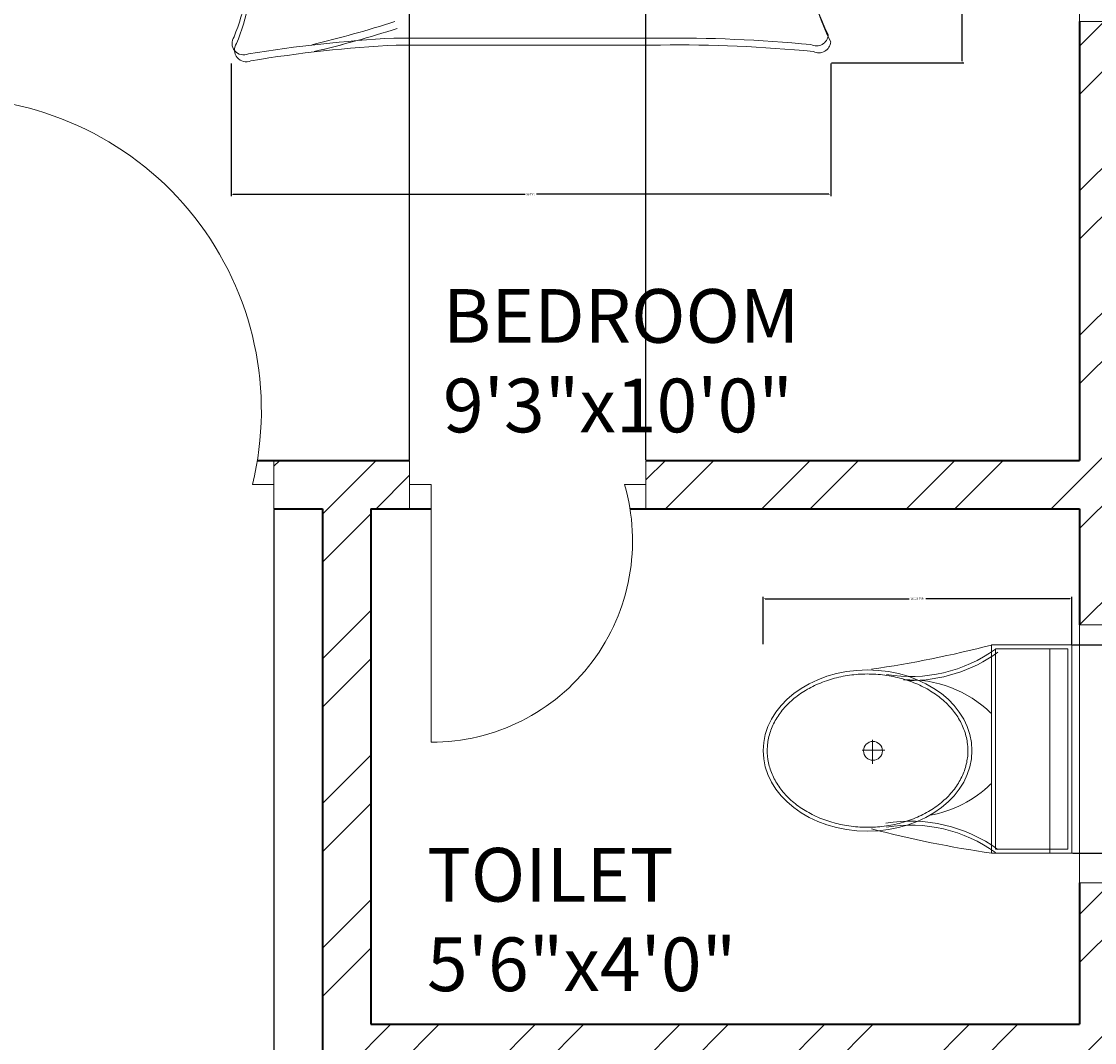
# Model space of a CAD drawing. Units: inches. Extents: x 2552 to 3217, y 1417 to 2737.
# Tile 23 of 25: x 3013 to 3113, y 2466 to 2561. Entities that reach past the tile are written whole.
import ezdxf

# ---------------------------------------------------------------- set-up
doc = ezdxf.new("R2010")
doc.units = ezdxf.units.IN
for name, color, linetype, lineweight in [('A-ANNO-DIMS', 2, 'Continuous', 18), ('A-AREA-IDEN', 7, 'Continuous', 18), ('A-DOOR', 21, 'Continuous', 18), ('A-FLOR-FIXT', 8, 'Continuous', 18), ('A-FURN', 8, 'Continuous', 13), ('A-GLAZ', 161, 'Continuous', 18), ('A-WALL', 7, 'Continuous', 35), ('A-WALL-PATT', 217, 'Continuous', 13)]:
    doc.layers.add(name, color=color, linetype=linetype, lineweight=lineweight)
doc.styles.get("Standard").update_dxf_attribs({"font": 'arial.ttf'})
doc.dimstyles.get("Standard").update_dxf_attribs({"dimtxt": 0.18, "dimasz": 0.18, "dimexe": 0.18, "dimexo": 0.0625, "dimgap": 0.09, "dimtad": 0, "dimtih": 1, "dimtoh": 1, "dimdec": 4, "dimzin": 0, "dimdsep": 46, "dimtxsty": 'Standard', "dimcen": 0.09, "dimadec": 0, "dimazin": 0, "dimtfac": 1, "dimtdec": 4, "dimtofl": 0, "dimtmove": 0, "dimatfit": 3, "dimfxl": 1, "dimtolj": 1, "dimtzin": 0, "dimarcsym": 0})

# ---------------------------------------------------------------- blocks, each defined once
blk = doc.blocks.new('A$C31115884')
for p, q in [((257.5, 466.4), (257.5, 523.2)), ((283.1, 497.7), (223.4, 497.7)), ((0, 200), (0, 0)), ((520, 200), (0, 200)), ((10, 190), (10, 10)), ((510, 190), (10, 190)), ((510, 10), (510, 190)), ((520, 0), (520, 200)), ((510, 54.5), (0, 54.5)), ((10, 10), (510, 10)), ((0, 0), (520, 0))]:
    blk.add_line(p, q)
blk.add_circle((255.6, 496.4), 23.6)
for centre, radius, start, end in [((2777.7, -204.6), 2807, 165.4549, 171.7133), ((3237, 905), 2807, 188.2867, 194.5451), ((-294.5, 403.3), 364.7, 324.2091, 9.3499), ((-294.5, 403.3), 374.7, 324.2091, 9.3499), ((805.8, 403.3), 364.7, 170.6501, 215.7909), ((139.5, 406.2), 293.5, 315.8436, 2.6563), ((805.8, 403.3), 374.7, 179.2036, 215.7909), ((383.6, 406.2), 293.5, 190.2774, 224.1564)]:
    blk.add_arc(centre, radius, start, end)
blk.add_ellipse((256.2, 509.9), major_axis=(0, -260.7), ratio=0.772727)
blk.add_open_spline([(256.2, 259.2), (263.1, 259.2), (270, 259.7), (287.8, 262.3), (298.7, 265.1), (319.9, 273.1), (330.2, 278.4), (350.1, 291.1), (359.7, 298.7), (377.7, 315.9), (386.2, 325.5), (401.7, 346.6), (408.8, 358.1), (421.3, 382.5), (426.8, 395.5), (435.9, 422.4), (439.5, 436.4), (444.8, 465.1), (446.5, 479.7), (447.9, 509.2), (447.6, 524), (445, 553.3), (442.7, 567.8), (436.3, 596), (432.1, 609.7), (421.9, 636), (416, 648.6), (402.5, 672.1), (395, 683), (378.6, 703), (369.8, 712.1), (351.1, 728), (341.3, 734.8), (320.9, 746.2), (310.4, 750.7), (288.9, 757.3), (278, 759.4), (256, 761), (245, 760.6), (223.1, 757.2), (212.3, 754.3), (191.1, 746.1), (180.8, 740.7), (160.9, 727.8), (151.4, 720.1), (133.5, 702.7), (125.1, 693), (109.6, 671.7), (102.6, 660.2), (90.2, 635.7), (84.9, 622.7), (76, 595.6), (72.4, 581.6), (67.2, 552.9), (65.6, 538.2), (64.4, 508.8), (64.8, 494), (67.5, 464.7), (69.9, 450.2), (76.6, 422), (80.8, 408.3), (91.1, 382.2), (97.2, 369.7), (110.8, 346.3), (118.4, 335.4), (134.8, 315.6), (143.7, 306.7), (162.4, 290.9), (172.3, 284.2), (192.8, 273), (203.3, 268.6), (224.8, 262.2), (235.8, 260.2), (249.9, 259.3), (253, 259.2), (256.2, 259.2)], degree=3, knots=[0, 0, 0, 0, 0.110105, 0.110105, 0.285049, 0.285049, 0.459994, 0.459994, 0.634938, 0.634938, 0.809882, 0.809882, 0.984827, 0.984827, 1.159771, 1.159771, 1.334715, 1.334715, 1.50966, 1.50966, 1.684604, 1.684604, 1.859549, 1.859549, 2.034493, 2.034493, 2.209437, 2.209437, 2.384382, 2.384382, 2.559326, 2.559326, 2.73427, 2.73427, 2.909215, 2.909215, 3.084159, 3.084159, 3.259103, 3.259103, 3.434048, 3.434048, 3.608992, 3.608992, 3.783936, 3.783936, 3.958881, 3.958881, 4.133825, 4.133825, 4.30877, 4.30877, 4.483714, 4.483714, 4.658658, 4.658658, 4.833603, 4.833603, 5.008547, 5.008547, 5.183491, 5.183491, 5.358436, 5.358436, 5.53338, 5.53338, 5.708324, 5.708324, 5.883269, 5.883269, 6.058213, 6.058213, 6.233158, 6.233158, 6.283185, 6.283185, 6.283185, 6.283185])
blk = doc.blocks.new('BED-DOUBLE')
for p, q in [((3.475, 63.333), (3.475, 81.443)), ((3.475, 63.333), (3.475, 81.443)), ((3.475, 81.443), (51.494, 81.443)), ((51.265, 81.443), (51.265, 54.833)), ((51.265, 81.443), (51.265, 54.833)), ((51.494, 81.443), (51.494, 80.804)), ((3.703, 62.694), (3.703, 80.804)), ((3.704, 62.694), (3.704, 80.804)), ((51.494, 80.804), (51.494, 54.194)), ((51.494, 80.804), (51.494, 54.194)), ((3.475, 79.91), (51.265, 79.91)), ((3.475, 79.91), (51.265, 79.91)), ((3.703, 79.27), (51.494, 79.27)), ((3.704, 79.27), (51.494, 79.27)), ((16.878, 78.416), (19.77, 79.139)), ((16.879, 78.416), (19.77, 79.139)), ((19.77, 79.139), (20.091, 79.139)), ((19.77, 79.139), (20.091, 79.139)), ((20.091, 79.139), (24.537, 78.995)), ((20.091, 79.139), (24.537, 78.995)), ((24.537, 78.995), (25.983, 79.573)), ((24.537, 78.995), (25.982, 79.573)), ((24.765, 78.355), (26.211, 78.934)), ((24.765, 78.355), (26.211, 78.934)), ((25.982, 79.573), (26.561, 74.223)), ((25.983, 79.573), (26.561, 74.223)), ((26.211, 78.934), (26.789, 73.584)), ((26.211, 78.934), (26.789, 73.584)), ((27.977, 78.951), (27.733, 73.576)), ((27.977, 78.952), (27.734, 73.576)), ((29.456, 78.464), (27.977, 78.952)), ((29.456, 78.464), (27.977, 78.951)), ((50.112, 78.886), (44.709, 78.983)), ((44.709, 78.983), (45.712, 78.901)), ((50.112, 78.886), (44.71, 78.983)), ((44.71, 78.983), (45.712, 78.901)), ((3.894, 78.127), (4.473, 74.946)), ((3.895, 78.127), (4.473, 74.946)), ((3.898, 78.105), (8.179, 78.435)), ((3.899, 78.105), (8.18, 78.435)), ((8.179, 78.435), (8.285, 78.416)), ((8.18, 78.435), (8.285, 78.416)), ((8.285, 78.416), (12.108, 78.127)), ((8.285, 78.416), (12.108, 78.127)), ((12.108, 78.127), (17.602, 77.115)), ((12.108, 78.127), (17.601, 77.115)), ((14.855, 77.693), (16.879, 78.416)), ((14.855, 77.693), (16.878, 78.416)), ((17.107, 77.777), (19.998, 78.5)), ((17.107, 77.777), (19.998, 78.5)), ((19.998, 78.5), (20.32, 78.5)), ((19.998, 78.5), (20.32, 78.5)), ((20.32, 78.5), (24.765, 78.355)), ((20.32, 78.5), (24.765, 78.355)), ((28.205, 78.312), (27.962, 72.937)), ((28.205, 78.312), (27.962, 72.937)), ((29.684, 77.825), (28.205, 78.312)), ((29.684, 77.825), (28.205, 78.312)), ((33.884, 78.886), (29.456, 78.464)), ((33.883, 78.886), (29.456, 78.464)), ((34.112, 78.247), (29.684, 77.825)), ((34.112, 78.247), (29.684, 77.825)), ((34.204, 78.906), (33.883, 78.886)), ((34.205, 78.906), (33.884, 78.886)), ((34.433, 78.267), (34.112, 78.247)), ((34.433, 78.267), (34.112, 78.247)), ((37.135, 78.365), (34.204, 78.906)), ((37.135, 78.365), (34.205, 78.906)), ((37.364, 77.726), (34.433, 78.267)), ((37.363, 77.726), (34.433, 78.267)), ((41.914, 78.374), (36.495, 77.021)), ((41.914, 78.374), (36.495, 77.021)), ((39.2, 77.77), (37.135, 78.365)), ((39.2, 77.77), (37.135, 78.365)), ((45.712, 78.901), (41.914, 78.374)), ((45.712, 78.901), (41.914, 78.374)), ((45.941, 78.262), (42.143, 77.735)), ((45.941, 78.262), (42.143, 77.735)), ((50.34, 78.247), (44.938, 78.344)), ((44.938, 78.344), (45.941, 78.262)), ((50.34, 78.247), (44.938, 78.344)), ((44.938, 78.344), (45.941, 78.262)), ((50.112, 78.886), (49.733, 75.675)), ((50.112, 78.886), (49.733, 75.675)), ((50.34, 78.247), (49.961, 75.036)), ((50.34, 78.247), (49.962, 75.036)), ((4.123, 77.488), (4.701, 74.307)), ((4.123, 77.488), (4.701, 74.307)), ((4.127, 77.466), (8.408, 77.795)), ((4.127, 77.466), (8.408, 77.795)), ((8.408, 77.795), (8.513, 77.777)), ((8.408, 77.795), (8.513, 77.777)), ((8.513, 77.777), (12.337, 77.488)), ((8.513, 77.777), (12.336, 77.488)), ((12.336, 77.488), (17.83, 76.476)), ((12.337, 77.488), (17.83, 76.476)), ((15.083, 77.054), (17.107, 77.777)), ((15.083, 77.054), (17.107, 77.777)), ((42.143, 77.735), (36.723, 76.382)), ((42.143, 77.735), (36.724, 76.382)), ((39.428, 77.13), (37.363, 77.726)), ((39.429, 77.13), (37.364, 77.726)), ((4.473, 74.946), (4.039, 72.344)), ((4.473, 74.946), (4.039, 72.344)), ((5.051, 72.488), (6.063, 75.235)), ((5.051, 72.488), (6.063, 75.235)), ((49.31, 73.186), (48.128, 75.865)), ((49.309, 73.186), (48.128, 75.865)), ((49.538, 72.547), (48.356, 75.226)), ((49.538, 72.547), (48.357, 75.226)), ((49.733, 75.675), (50.329, 73.105)), ((49.733, 75.675), (50.328, 73.105)), ((49.961, 75.036), (50.557, 72.466)), ((49.962, 75.036), (50.557, 72.466)), ((4.701, 74.307), (4.267, 71.704)), ((4.701, 74.307), (4.268, 71.704)), ((5.279, 71.849), (6.291, 74.596)), ((5.28, 71.849), (6.291, 74.596)), ((26.561, 74.223), (27.139, 71.042)), ((26.561, 74.223), (27.139, 71.042)), ((26.789, 73.584), (27.367, 70.403)), ((26.789, 73.584), (27.367, 70.403)), ((27.734, 73.576), (27.355, 70.365)), ((27.733, 73.576), (27.355, 70.365)), ((27.962, 72.937), (27.583, 69.726)), ((27.962, 72.937), (27.583, 69.726)), ((50.112, 69.615), (49.309, 73.186)), ((50.112, 69.615), (49.31, 73.186)), ((50.328, 73.105), (49.814, 72.059)), ((50.329, 73.105), (49.815, 72.059)), ((4.039, 72.344), (4.618, 71.332)), ((4.039, 72.344), (4.617, 71.332)), ((4.473, 68.874), (5.051, 72.488)), ((4.473, 68.874), (5.051, 72.488)), ((50.341, 68.975), (49.538, 72.547)), ((50.34, 68.975), (49.538, 72.547)), ((50.557, 72.466), (50.043, 71.419)), ((50.557, 72.466), (50.043, 71.419)), ((4.267, 71.704), (4.846, 70.692)), ((4.268, 71.704), (4.846, 70.692)), ((4.701, 68.234), (5.28, 71.849)), ((4.701, 68.234), (5.279, 71.849)), ((27.139, 71.042), (27.139, 69.741)), ((27.139, 71.042), (27.139, 69.741)), ((27.355, 70.365), (27.436, 69.067)), ((27.355, 70.365), (27.436, 69.067)), ((27.367, 70.403), (27.367, 69.102)), ((27.367, 70.403), (27.367, 69.102)), ((27.139, 69.741), (26.561, 67.861)), ((27.139, 69.741), (26.561, 67.861)), ((27.367, 69.102), (26.789, 67.222)), ((27.367, 69.102), (26.789, 67.222)), ((27.436, 69.067), (28.13, 67.227)), ((27.436, 69.067), (28.13, 67.227)), ((27.583, 69.726), (27.664, 68.427)), ((27.583, 69.726), (27.664, 68.427)), ((49.923, 68.009), (50.112, 69.615)), ((49.923, 68.009), (50.112, 69.615)), ((50.151, 67.37), (50.341, 68.975)), ((50.151, 67.37), (50.34, 68.975)), ((4.762, 67.283), (4.473, 68.874)), ((4.762, 67.283), (4.473, 68.874)), ((4.99, 66.644), (4.701, 68.234)), ((4.99, 66.644), (4.701, 68.234)), ((27.664, 68.427), (28.359, 66.587)), ((27.664, 68.427), (28.359, 66.587)), ((50.698, 64.871), (49.923, 68.009)), ((50.698, 64.871), (49.923, 68.009)), ((4.184, 64.102), (4.762, 67.283)), ((4.184, 64.102), (4.762, 67.283)), ((26.561, 67.861), (26.561, 65.18)), ((26.561, 67.861), (26.561, 65.18)), ((26.789, 67.222), (26.789, 64.541)), ((26.789, 67.222), (26.789, 64.541)), ((28.13, 67.227), (28.298, 64.55)), ((28.13, 67.227), (28.297, 64.55)), ((50.927, 64.231), (50.151, 67.37)), ((50.926, 64.231), (50.151, 67.37)), ((4.412, 63.463), (4.99, 66.644)), ((4.412, 63.463), (4.99, 66.644)), ((24.103, 65.18), (20.959, 66.271)), ((24.103, 65.18), (20.959, 66.271)), ((28.359, 66.587), (28.526, 63.911)), ((28.359, 66.587), (28.526, 63.911)), ((30.75, 64.704), (33.821, 65.989)), ((30.75, 64.704), (33.821, 65.989)), ((6.381, 65.815), (10.413, 65.148)), ((6.382, 65.815), (10.414, 65.148)), ((6.61, 65.175), (10.642, 64.509)), ((6.61, 65.175), (10.642, 64.509)), ((10.413, 65.148), (9.28, 64.825)), ((10.414, 65.148), (9.281, 64.825)), ((10.413, 65.148), (17.423, 64.717)), ((10.414, 65.148), (17.424, 64.717)), ((17.423, 64.717), (19.384, 65.274)), ((17.424, 64.717), (19.384, 65.274)), ((19.384, 65.274), (24.516, 64.871)), ((19.384, 65.274), (24.516, 64.871)), ((24.332, 64.541), (21.187, 65.632)), ((24.332, 64.541), (21.187, 65.632)), ((26.561, 65.18), (24.103, 65.18)), ((26.561, 65.18), (24.103, 65.18)), ((30.978, 64.064), (34.049, 65.349)), ((30.979, 64.064), (34.049, 65.349)), ((32.564, 65.815), (36.596, 65.148)), ((32.564, 65.815), (36.596, 65.148)), ((32.792, 65.175), (36.824, 64.509)), ((32.793, 65.175), (36.825, 64.509)), ((36.596, 65.148), (43.606, 64.717)), ((36.596, 65.148), (43.606, 64.717)), ((43.606, 64.717), (45.567, 65.274)), ((43.606, 64.717), (45.566, 65.274)), ((45.566, 65.274), (50.698, 64.871)), ((45.567, 65.274), (50.698, 64.871)), ((9.281, 64.825), (4.184, 64.102)), ((9.28, 64.825), (4.184, 64.102)), ((9.509, 64.186), (4.412, 63.463)), ((9.509, 64.186), (4.412, 63.463)), ((10.642, 64.509), (9.509, 64.186)), ((10.642, 64.509), (9.509, 64.186)), ((10.642, 64.509), (17.652, 64.078)), ((10.642, 64.509), (17.652, 64.078)), ((17.652, 64.078), (19.612, 64.635)), ((17.652, 64.078), (19.612, 64.635)), ((19.612, 64.635), (24.744, 64.231)), ((19.612, 64.635), (24.744, 64.231)), ((26.789, 64.541), (24.332, 64.541)), ((26.789, 64.541), (24.332, 64.541)), ((28.297, 64.55), (30.75, 64.704)), ((28.298, 64.55), (30.75, 64.704)), ((28.526, 63.911), (30.979, 64.064)), ((28.526, 63.911), (30.978, 64.064)), ((30.259, 64.06), (34.449, 57.567)), ((30.259, 64.06), (34.449, 57.567)), ((40.644, 61.127), (32.306, 64.06)), ((40.644, 61.127), (32.306, 64.06)), ((36.824, 64.509), (43.834, 64.078)), ((36.825, 64.509), (43.835, 64.078)), ((43.834, 64.078), (45.795, 64.635)), ((43.835, 64.078), (45.795, 64.635)), ((45.795, 64.635), (50.927, 64.231)), ((45.795, 64.635), (50.926, 64.231)), ((30.487, 63.421), (34.677, 56.927)), ((30.488, 63.421), (34.678, 56.927)), ((40.872, 60.487), (32.534, 63.421)), ((40.873, 60.487), (32.535, 63.421)), ((46.22, 59.115), (40.644, 61.127)), ((46.219, 59.115), (40.644, 61.127)), ((46.448, 58.475), (40.872, 60.487)), ((46.448, 58.475), (40.873, 60.487)), ((49.162, 56.948), (46.219, 59.115)), ((49.162, 56.948), (46.22, 59.115)), ((49.391, 56.308), (46.448, 58.475)), ((49.39, 56.308), (46.448, 58.475)), ((34.449, 57.567), (36.153, 53.078)), ((34.449, 57.567), (36.153, 53.078)), ((34.677, 56.927), (36.381, 52.439)), ((34.678, 56.927), (36.381, 52.439)), ((52.868, 53.697), (49.162, 56.948)), ((52.867, 53.697), (49.162, 56.948)), ((53.096, 53.058), (49.39, 56.308)), ((53.096, 53.058), (49.391, 56.308)), ((36.153, 53.078), (36.463, 51.066)), ((36.153, 53.078), (36.462, 51.066)), ((40.954, 52.614), (44.361, 53.078)), ((40.954, 52.614), (44.361, 53.078)), ((44.361, 53.078), (48.233, 53.388)), ((44.361, 53.078), (48.233, 53.388)), ((48.233, 53.388), (51.331, 53.078)), ((48.233, 53.388), (51.33, 53.078)), ((51.33, 53.078), (52.867, 53.697)), ((51.331, 53.078), (52.868, 53.697)), ((51.559, 52.439), (53.096, 53.058)), ((51.559, 52.439), (53.096, 53.058)), ((52.947, 51.953), (52.867, 53.697, 3.871)), ((52.947, 51.953), (52.868, 53.697, 3.871)), ((53.176, 51.313), (53.096, 53.058, 3.871)), ((53.175, 51.313), (53.096, 53.058, 3.871)), ((36.381, 52.439), (36.691, 50.427)), ((36.381, 52.439), (36.691, 50.427)), ((38.94, 51.685), (40.954, 52.614)), ((38.941, 51.685), (40.954, 52.614)), ((39.169, 51.046), (41.182, 51.975)), ((39.169, 51.046), (41.182, 51.975)), ((41.182, 51.975), (44.59, 52.439)), ((41.182, 51.975), (44.589, 52.439)), ((44.589, 52.439), (48.461, 52.748)), ((44.59, 52.439), (48.461, 52.748)), ((48.461, 52.748), (51.559, 52.439)), ((48.461, 52.748), (51.559, 52.439)), ((36.462, 51.066), (38.94, 51.685)), ((36.463, 51.066), (38.941, 51.685)), ((36.691, 50.427), (39.169, 51.046)), ((36.691, 50.427), (39.169, 51.046)), ((15.063, 2.198), (39.677, 2.198)), ((15.063, 2.198), (39.677, 2.198)), ((15.292, 1.559), (39.906, 1.559)), ((15.292, 1.559), (39.905, 1.559))]:
    blk.add_line(p, q)
for centre, radius, start, end in [((21.359, -100.609), 164.969, 86.08655, 96.78213), ((21.359, -100.609), 164.969, 86.08655, 96.78213), ((85.162, 61.347), 83.306, 178.72178, 185.60397), ((85.162, 61.347), 83.306, 178.72178, 185.60397), ((21.587, -101.249), 164.969, 86.08655, 96.78213), ((21.587, -101.249), 164.969, 86.08655, 96.78213), ((85.39, 60.708), 83.306, 178.72178, 185.60397), ((85.39, 60.708), 83.306, 178.72178, 185.60397), ((17.756, -74.873), 129.02, 81.78449, 96.90062), ((17.756, -74.873), 129.02, 81.78449, 96.90062), ((17.984, -75.512), 129.02, 81.78449, 96.90062), ((17.984, -75.512), 129.02, 81.78449, 96.90062), ((-167.307, 50.27), 170.11, 358.4762, 1.00819), ((-167.308, 50.27), 170.11, 358.4762, 1.00819), ((-167.079, 49.63), 170.11, 358.4762, 1.00819), ((-167.079, 49.63), 170.11, 358.4762, 1.00819), ((31.154, 79.961), 29.654, 280.66171, 289.88058), ((31.154, 79.961), 29.654, 280.66171, 289.88058), ((43.744, 46.377), 6.224, 78.6608, 113.73842), ((43.743, 46.377), 6.224, 78.6608, 113.73842), ((43.972, 45.738), 6.224, 78.6608, 113.73842), ((43.972, 45.738), 6.224, 78.6608, 113.73842), ((51.327, 88.099), 36.183, 259.87628, 272.56571), ((51.327, 88.099), 36.183, 259.87628, 272.56571), ((36.636, 51.004), 0.185, 160.24637, 271.13765), ((36.636, 51.004), 0.185, 160.24637, 271.13765), ((31.382, 79.322), 29.654, 280.66171, 289.88058), ((31.382, 79.322), 29.654, 280.66171, 289.88058), ((51.555, 87.46), 36.183, 259.87628, 272.56571), ((51.556, 87.46), 36.183, 259.87628, 272.56571), ((182.266, 45.128), 129.499, 176.97912, 183.83645), ((182.266, 45.128), 129.499, 176.97912, 183.83645), ((182.494, 44.489), 129.499, 176.97912, 183.83645), ((182.494, 44.489), 129.499, 176.97912, 183.83645), ((36.865, 50.365), 0.185, 160.24637, 271.13765), ((36.864, 50.365), 0.185, 160.24637, 271.13765), ((484.822, 30.829), 482.31, 178.22771, 181.71854), ((484.822, 30.829), 482.31, 178.22771, 181.71854), ((485.051, 30.19), 482.31, 178.22771, 181.71854), ((485.051, 30.19), 482.31, 178.22771, 181.71854), ((-4508.743, 13.622), 4561.858, 0.002168, 0.286887), ((-4508.744, 13.622), 4561.858, 0.002168, 0.286887), ((-4508.515, 12.983), 4561.858, 0.002168, 0.286887), ((-4508.515, 12.983), 4561.858, 0.002168, 0.286887), ((-26.899, 16.928), 29.634, 346.06484, 358.91125), ((-26.9, 16.928), 29.634, 346.06484, 358.91125), ((-26.671, 16.289), 29.634, 346.06484, 358.91125), ((-26.671, 16.289), 29.634, 346.06484, 358.91125), ((76.157, 12.777), 23.065, 177.47136, 206.46809), ((76.157, 12.777), 23.065, 177.47136, 206.46809), ((76.386, 12.138), 23.065, 177.47136, 206.46809), ((76.385, 12.138), 23.065, 177.47136, 206.46809), ((-21.659, 11.168), 23.562, 337.97508, 356.652), ((-21.66, 11.168), 23.562, 337.97508, 356.652), ((-21.431, 10.528), 23.562, 337.97508, 356.652), ((-21.431, 10.528), 23.562, 337.97508, 356.652), ((-17.222, 105.155), 106.459, 283.38322, 287.70533), ((-17.222, 105.155), 106.459, 283.38322, 287.70533), ((-16.993, 104.516), 106.459, 283.38322, 287.70533), ((-16.994, 104.516), 106.459, 283.38322, 287.70533), ((1.087, 1.725), 1.089, 146.17358, 293.47814), ((1.088, 1.725), 1.089, 146.17358, 293.47814), ((21.427, -119.394), 121.759, 92.99578, 99.40907), ((21.427, -119.394), 121.759, 92.99578, 99.40907), ((41.152, -130.833), 133.04, 84.4998, 90.63509), ((41.152, -130.833), 133.04, 84.4998, 90.63509), ((54.41, 2.573), 1.102, 242.65876, 356.02002), ((54.41, 2.573), 1.102, 242.65876, 356.02002), ((1.316, 1.086), 1.089, 146.17358, 293.47814), ((1.316, 1.086), 1.089, 146.17358, 293.47814), ((21.655, -120.033), 121.759, 92.99578, 99.40907), ((21.655, -120.033), 121.759, 92.99578, 99.40907), ((41.38, -131.473), 133.04, 84.4998, 90.63509), ((41.38, -131.473), 133.04, 84.4998, 90.63509), ((54.638, 1.934), 1.102, 242.65876, 356.02002), ((54.638, 1.934), 1.102, 242.65876, 356.02002)]:
    blk.add_arc(centre, radius, start, end)
blk = doc.blocks.new('WIN-48')
for p, q in [((4.5, 48), (0, 48)), ((0, 48), (9, 48)), ((0, 48), (0, 0)), ((4.5, 0), (4.5, 48)), ((9, 48), (9, 0)), ((0, 0), (9, 0)), ((9, 0), (4.5, 0))]:
    blk.add_line(p, q)
blk = doc.blocks.new('WIN-24')
for p, q in [((0, 24), (9, 24)), ((0, 24), (0, 0)), ((9, 24), (4.5, 24)), ((4.5, 24), (4.5, 0)), ((9, 24), (9, 0)), ((4.5, 0), (0, 0)), ((0, 0), (9, 0))]:
    blk.add_line(p, q)
blk = doc.blocks.new('*D17')
at = {"layer": 'A-ANNO-DIMS', "color": 0, "lineweight": -2, "transparency": 16777216}
for p, q in [((3081.899, 2503.385), (3081.899, 2507.811)), ((3110.619, 2503.385), (3110.619, 2507.811)), ((3082.079, 2507.631), (3095.483, 2507.631)), ((3110.439, 2507.631), (3097.035, 2507.631))]:
    blk.add_line(p, q, dxfattribs=at)
at = {"layer": 'A-ANNO-DIMS', "color": 0, "transparency": 16777216}
for points in [[(3082.079, 2507.661), (3082.079, 2507.601), (3081.899, 2507.631)], [(3110.439, 2507.661), (3110.439, 2507.601), (3110.619, 2507.631)]]:
    blk.add_solid(points, dxfattribs=at)
at = {"layer": 'Defpoints', "color": 0, "transparency": 16777216}
for p in [(3081.899, 2507.631), (3081.899, 2503.323), (3110.619, 2503.323)]:
    blk.add_point(p, dxfattribs=at)
at = {"layer": 'A-ANNO-DIMS', "color": 0, "transparency": 16777216, "insert": (3096.259, 2507.631), "char_height": 0.18, "attachment_point": 5}
blk.add_mtext('\\A1;WC 29 TYP.', dxfattribs=at)
blk = doc.blocks.new('*D18')
at = {"layer": 'A-ANNO-DIMS', "color": 0, "lineweight": -2, "transparency": 16777216}
for p, q in [((3110.682, 2503.323), (3115.108, 2503.323)), ((3114.928, 2503.143), (3114.928, 2493.814)), ((3114.928, 2484.122), (3114.928, 2493.45)), ((3110.682, 2483.942), (3115.108, 2483.942))]:
    blk.add_line(p, q, dxfattribs=at)
at = {"layer": 'A-ANNO-DIMS', "color": 0, "transparency": 16777216}
for points in [[(3114.898, 2503.143), (3114.958, 2503.143), (3114.928, 2503.323)], [(3114.898, 2484.122), (3114.958, 2484.122), (3114.928, 2483.942)]]:
    blk.add_solid(points, dxfattribs=at)
at = {"layer": 'Defpoints', "color": 0, "transparency": 16777216}
for p in [(3110.619, 2503.323), (3114.928, 2503.323), (3110.619, 2483.942)]:
    blk.add_point(p, dxfattribs=at)
at = {"layer": 'A-ANNO-DIMS', "color": 0, "transparency": 16777216, "insert": (3114.928, 2493.632), "char_height": 0.18, "attachment_point": 5}
blk.add_mtext('\\A1;19 TYP.', dxfattribs=at)
blk = doc.blocks.new('*D19')
at = {"layer": 'A-ANNO-DIMS', "color": 0, "lineweight": -2, "transparency": 16777216}
for p, q in [((3088.244, 2639.06), (3100.593, 2639.06)), ((3100.413, 2638.88), (3100.413, 2598.468)), ((3100.413, 2557.691), (3100.413, 2598.104)), ((3088.244, 2557.511), (3100.593, 2557.511))]:
    blk.add_line(p, q, dxfattribs=at)
at = {"layer": 'A-ANNO-DIMS', "color": 0, "transparency": 16777216}
for points in [[(3100.383, 2638.88), (3100.443, 2638.88), (3100.413, 2639.06)], [(3100.383, 2557.691), (3100.443, 2557.691), (3100.413, 2557.511)]]:
    blk.add_solid(points, dxfattribs=at)
at = {"layer": 'Defpoints', "color": 0, "transparency": 16777216}
for p in [(3088.181, 2639.06), (3100.413, 2639.06), (3088.181, 2557.511)]:
    blk.add_point(p, dxfattribs=at)
at = {"layer": 'A-ANNO-DIMS', "color": 0, "transparency": 16777216, "insert": (3100.413, 2598.286), "char_height": 0.18, "attachment_point": 5}
blk.add_mtext('\\A1;BED 82 TYP.', dxfattribs=at)
blk = doc.blocks.new('*D20')
at = {"layer": 'A-ANNO-DIMS', "color": 0, "lineweight": -2, "transparency": 16777216}
for p, q in [((3032.356, 2557.449), (3032.356, 2545.099)), ((3088.181, 2557.449), (3088.181, 2545.099)), ((3032.536, 2545.279), (3059.741, 2545.279)), ((3088.001, 2545.279), (3060.797, 2545.279))]:
    blk.add_line(p, q, dxfattribs=at)
at = {"layer": 'A-ANNO-DIMS', "color": 0, "transparency": 16777216}
for points in [[(3032.536, 2545.309), (3032.536, 2545.249), (3032.356, 2545.279)], [(3088.001, 2545.309), (3088.001, 2545.249), (3088.181, 2545.279)]]:
    blk.add_solid(points, dxfattribs=at)
at = {"layer": 'Defpoints', "color": 0, "transparency": 16777216}
for p in [(3032.356, 2557.511), (3088.181, 2557.511), (3088.181, 2545.279)]:
    blk.add_point(p, dxfattribs=at)
at = {"layer": 'A-ANNO-DIMS', "color": 0, "transparency": 16777216, "insert": (3060.269, 2545.279), "char_height": 0.18, "attachment_point": 5}
blk.add_mtext('\\A1;56 TYP.', dxfattribs=at)
blk = doc.blocks.new('*D57')
at = {"layer": 'A-ANNO-DIMS', "color": 0, "lineweight": -2, "transparency": 16777216}
for p, q in [((3004.084, 2515.95), (3004.084, 1482.533)), ((3036.34, 2515.95), (3036.34, 1482.533)), ((3004.264, 1482.713), (3019.748, 1482.713)), ((3036.16, 1482.713), (3020.676, 1482.713))]:
    blk.add_line(p, q, dxfattribs=at)
at = {"layer": 'A-ANNO-DIMS', "color": 0, "transparency": 16777216}
for points in [[(3004.264, 1482.743), (3004.264, 1482.683), (3004.084, 1482.713)], [(3036.16, 1482.743), (3036.16, 1482.683), (3036.34, 1482.713)]]:
    blk.add_solid(points, dxfattribs=at)
at = {"layer": 'Defpoints', "color": 0, "transparency": 16777216}
for p in [(3004.084, 2516.013), (3036.34, 2516.013), (3036.34, 1482.713)]:
    blk.add_point(p, dxfattribs=at)
at = {"layer": 'A-ANNO-DIMS', "color": 0, "transparency": 16777216, "insert": (3020.212, 1482.713), "char_height": 0.18, "attachment_point": 5}
blk.add_mtext('\\A1;32.255', dxfattribs=at)
blk = doc.blocks.new('*D58')
at = {"layer": 'A-ANNO-DIMS', "color": 0, "lineweight": -2, "transparency": 16777216}
for p, q in [((3048.979, 2520.575), (3048.979, 2709.493)), ((3049.159, 2709.313), (3059.515, 2709.313)), ((3070.801, 2709.313), (3060.445, 2709.313)), ((3070.981, 2520.575), (3070.981, 2709.493))]:
    blk.add_line(p, q, dxfattribs=at)
at = {"layer": 'A-ANNO-DIMS', "color": 0, "transparency": 16777216}
for points in [[(3049.159, 2709.343), (3049.159, 2709.283), (3048.979, 2709.313)], [(3070.801, 2709.343), (3070.801, 2709.283), (3070.981, 2709.313)]]:
    blk.add_solid(points, dxfattribs=at)
at = {"layer": 'Defpoints', "color": 0, "transparency": 16777216}
for p in [(3070.981, 2709.313), (3048.979, 2520.513), (3070.981, 2520.513)]:
    blk.add_point(p, dxfattribs=at)
at = {"layer": 'A-ANNO-DIMS', "color": 0, "transparency": 16777216, "insert": (3059.98, 2709.313), "char_height": 0.18, "attachment_point": 5}
blk.add_mtext('\\A1;22.003', dxfattribs=at)
blk = doc.blocks.new('*D66')
at = {"layer": 'A-ANNO-DIMS', "color": 0, "lineweight": -2, "transparency": 16777216}
for p, q in [((3120.416, 2481.184), (3180.334, 2481.184)), ((3180.154, 2481.004), (3180.154, 2434.28)), ((3180.154, 2387.193), (3180.154, 2433.916)), ((3111.416, 2387.013), (3180.334, 2387.013))]:
    blk.add_line(p, q, dxfattribs=at)
at = {"layer": 'A-ANNO-DIMS', "color": 0, "transparency": 16777216}
for points in [[(3180.124, 2481.004), (3180.184, 2481.004), (3180.154, 2481.184)], [(3180.124, 2387.193), (3180.184, 2387.193), (3180.154, 2387.013)]]:
    blk.add_solid(points, dxfattribs=at)
at = {"layer": 'Defpoints', "color": 0, "transparency": 16777216}
for p in [(3120.354, 2481.184), (3111.354, 2387.013), (3180.154, 2387.013)]:
    blk.add_point(p, dxfattribs=at)
at = {"layer": 'A-ANNO-DIMS', "color": 0, "transparency": 16777216, "insert": (3180.154, 2434.098), "char_height": 0.18, "attachment_point": 5}
blk.add_mtext('\\A1;94.17', dxfattribs=at)

msp = doc.modelspace()

# ---------------------------------------------------------------- hatches: boundary and pattern name
at = {"layer": 'A-WALL-PATT'}
h = msp.add_hatch(dxfattribs=at)
h.set_pattern_fill('ANSI32', color=256)
h.paths.add_polyline_path([(2756.676, 2649.5125), (2637.3535, 2649.5125), (2637.3535, 2617.9626), (2641.8535, 2617.9626), (2646.3535, 2617.9626), (2646.3535, 2640.5125), (2724.3535, 2640.5125), (2724.3535, 2520.5125), (2720.299, 2520.5125), (2720.299, 2516.0125), (2733.4075, 2516.0125), (2733.4075, 2518.2213), (2733.4075, 2520.5125), (2728.8535, 2520.5125), (2728.8535, 2640.5125), (2756.676, 2640.5125)])
h.paths.add_polyline_path([(2848.8535, 2649.5125), (2804.676, 2649.5125), (2804.676, 2640.5125), (2839.8535, 2640.5125), (2839.8535, 2598.3517), (2848.8535, 2598.3517)])
h.paths.add_polyline_path([(2646.3535, 2516.0125), (2697.9593, 2516.0125), (2697.9593, 2518.2625), (2697.9593, 2520.5125), (2646.3535, 2520.5125), (2646.3535, 2581.9626), (2637.3535, 2581.9626), (2637.3535, 2364.3298), (2646.3535, 2364.3298), (2646.3535, 2387.0125), (2724.3535, 2387.0125), (2724.3535, 2267.0125), (2721.0443, 2267.0125), (2721.0443, 2262.5125), (2733.7854, 2262.5125), (2733.7854, 2264.7625), (2733.7854, 2267.0125), (2728.8535, 2267.0125), (2728.8535, 2387.0125), (2839.8535, 2387.0125), (2839.8535, 2363.8387), (2848.8535, 2363.8387), (2848.8535, 2403.7415), (2844.3535, 2403.7415), (2839.8535, 2403.7415), (2839.8535, 2396.0125), (2646.3535, 2396.0125)])
h.paths.add_polyline_path([(2848.8535, 2550.3517), (2844.3535, 2550.3517), (2839.8535, 2550.3517), (2839.8535, 2520.5125), (2801.9195, 2520.5125), (2801.9195, 2518.2625), (2801.9195, 2516.0125), (2839.8535, 2516.0125), (2839.8535, 2507.5813), (2848.8535, 2507.5813)], flags=17)
h.paths.add_polyline_path([(2848.8535, 2483.5813), (2844.3535, 2483.5813), (2839.8535, 2483.5813), (2839.8535, 2468.0125), (2773.8535, 2468.0125), (2773.8535, 2516.0125), (2778.1336, 2516.0125), (2778.1336, 2520.5125), (2766.696, 2520.5125), (2766.696, 2518.2625), (2766.696, 2516.0125), (2769.3535, 2516.0125), (2769.3535, 2463.5125), (2839.8535, 2463.5125), (2839.8535, 2431.0782), (2848.8535, 2431.0782)], flags=17)
h.paths.add_polyline_path([(2917.8535, 2569.2764), (2913.3535, 2569.2764), (2908.8535, 2569.2764), (2908.8535, 2433.001), (2917.8535, 2433.001), (2917.8535, 2516.0125), (2967.486, 2516.0125), (2967.486, 2520.5125), (2917.8535, 2520.5125)])
h.paths.add_polyline_path([(3000.3535, 2640.5125), (2995.8535, 2640.5125), (2995.8535, 2520.5125), (2990.688, 2520.5125), (2990.688, 2516.0125), (3004.0844, 2516.0125), (3004.0844, 2518.2625), (3004.0844, 2520.5125), (3000.3535, 2520.5125)])
h.paths.add_polyline_path([(3120.3535, 2561.3689), (3115.8535, 2561.3689), (3111.3535, 2561.3689), (3111.3535, 2520.5125), (3070.9814, 2520.5125), (3070.9814, 2518.2625), (3070.9814, 2516.0125), (3111.3535, 2516.0125), (3111.3535, 2505.1841), (3120.3535, 2505.1841)])
h.paths.add_polyline_path([(3120.3535, 2481.1841), (3115.8535, 2481.1841), (3111.3535, 2481.1841), (3111.3535, 2468.0125), (3045.3535, 2468.0125), (3045.3535, 2516.0125), (3048.9787, 2516.0125), (3048.9787, 2520.5125), (3036.3395, 2520.5125), (3036.3395, 2516.0125), (3040.8535, 2516.0125), (3040.8535, 2463.5125), (3111.3535, 2463.5125), (3111.3535, 2396.0125), (2917.8535, 2396.0125), (2917.8535, 2403.4124), (2913.3535, 2403.4124), (2908.8535, 2403.4124), (2908.8535, 2182.5756), (2917.8535, 2182.5756), (2917.8535, 2262.5125), (2968.001, 2262.5125), (2968.001, 2264.7625), (2968.001, 2267.0125), (2917.8535, 2267.0125), (2917.8535, 2387.0125), (3111.3535, 2387.0125), (3111.3535, 2352.2435), (3120.3535, 2352.2435)])
h.paths.add_polyline_path([(3120.3535, 2304.2435), (3115.8535, 2304.2435), (3111.3535, 2304.2435), (3111.3535, 2267.0125), (3073.8616, 2267.0125), (3073.8616, 2264.7625), (3073.8616, 2262.5125), (3111.3535, 2262.5125), (3111.3535, 2252.376), (3120.3535, 2252.376)], flags=17)
h.paths.add_polyline_path([(3120.3535, 2228.376), (3115.8535, 2228.376), (3111.3535, 2228.376), (3111.3535, 2214.5125), (3045.3535, 2214.5125), (3045.3535, 2262.5125), (3049.3096, 2262.5125), (3049.3096, 2267.0125), (3035.0125, 2267.0125), (3035.0125, 2262.5125), (3040.8535, 2262.5125), (3040.8535, 2210.0125), (3111.3535, 2210.0125), (3111.3535, 2142.5125), (2917.8535, 2142.5125), (2917.8535, 2150.2408), (2913.3535, 2150.2408), (2908.8535, 2150.2408), (2908.8535, 1924.9905), (2917.8535, 1924.9905), (2917.8535, 2009.0125), (2971.959, 2009.0125), (2971.959, 2011.2625), (2971.959, 2013.5125), (2917.8535, 2013.5125), (2917.8535, 2133.5125), (2995.8535, 2133.5125), (2995.8535, 2013.5125), (2992.1797, 2013.5125), (2992.1797, 2009.0125), (3004.3344, 2009.0125), (3004.3344, 2011.2625), (3004.3344, 2013.5125), (3000.3535, 2013.5125), (3000.3535, 2133.5125), (3111.3535, 2133.5125), (3111.3535, 2115.0291), (3120.3535, 2115.0291)])
h.paths.add_polyline_path([(3000.3535, 2387.0125), (2995.8535, 2387.0125), (2995.8535, 2267.0125), (2991.3326, 2267.0125), (2991.3326, 2262.5125), (3004.1044, 2262.5125), (3004.1044, 2264.7625), (3004.1044, 2267.0125), (3000.3535, 2267.0125)], flags=17)
h.paths.add_polyline_path([(3120.3535, 1973.2388), (3115.8535, 1973.2388), (3111.3535, 1973.2388), (3111.3535, 1961.0125), (3045.3535, 1961.0125), (3045.3535, 2009.0125), (3048.9101, 2009.0125), (3048.9101, 2013.5125), (3037.105, 2013.5125), (3037.105, 2011.2625), (3037.105, 2009.0125), (3040.8535, 2009.0125), (3040.8535, 1956.5125), (3111.3535, 1956.5125), (3111.3535, 1889.0125), (2917.8535, 1889.0125), (2917.8535, 1895.7215), (2913.3535, 1895.7215), (2908.8535, 1895.7215), (2908.8535, 1844.2217), (2917.8535, 1844.2217), (2917.8535, 1880.0125), (3111.3535, 1880.0125), (3111.3535, 1846.9541), (3120.3535, 1846.9541)])
h.paths.add_polyline_path([(3120.3535, 2067.0291), (3111.3535, 2067.0291), (3111.3535, 2013.5125), (3071.3001, 2013.5125), (3071.3001, 2009.0125), (3111.3535, 2009.0125), (3111.3535, 1997.2388), (3120.3535, 1997.2388)], flags=0)
h.paths.add_polyline_path([(3120.3535, 1798.9541), (3115.8535, 1798.9541), (3111.3535, 1798.9541), (3111.3535, 1760.0125), (3071.2497, 1760.0125), (3071.2497, 1757.7625), (3071.2497, 1755.5125), (3111.3535, 1755.5125), (3111.3535, 1746.162), (3120.3535, 1746.2478)])
h.paths.add_polyline_path([(3120.3535, 1722.2049), (3111.3535, 1722.2049), (3111.3535, 1707.5125), (3045.3535, 1707.5125), (3045.3535, 1755.5125), (3048.6624, 1755.5125), (3048.6624, 1760.0125), (3035.3703, 1760.0125), (3035.3703, 1755.5125), (3040.8535, 1755.5125), (3040.8535, 1703.0125), (3111.3535, 1703.0125), (3111.3535, 1635.5125), (2917.8535, 1635.5125), (2917.8535, 1643.1366), (2913.3535, 1643.1366), (2908.8535, 1643.1366), (2908.8535, 1626.5125), (3120.3535, 1626.5125)])
h.paths.add_polyline_path([(2917.8535, 1755.5125), (2973.2287, 1755.5125), (2973.2287, 1757.7625), (2973.2287, 1760.0125), (2917.8535, 1760.0125), (2917.8535, 1808.2217), (2913.3535, 1808.2217), (2908.8535, 1808.2217), (2908.8535, 1676.1665), (2917.8535, 1676.1665)])
h.paths.add_polyline_path([(3000.3535, 1880.0125), (2995.8535, 1880.0125), (2995.8535, 1760.0125), (2992.9329, 1760.0125), (2992.9329, 1755.5125), (3003.8766, 1755.5125), (3003.8766, 1757.7625), (3003.8766, 1760.0125), (3000.3535, 1760.0125)])
h.paths.add_polyline_path([(2848.8535, 1896.6971), (2844.3535, 1896.6971), (2839.8535, 1896.6971), (2839.8535, 1889.0125), (2646.3535, 1889.0125), (2646.3535, 2009.0125), (2700.5253, 2009.0125), (2700.5253, 2011.2625), (2700.5253, 2013.5125), (2646.3535, 2013.5125), (2646.3535, 2053.1812), (2641.8535, 2053.1812), (2637.3535, 2053.1812), (2637.3535, 1836.254), (2646.3535, 1836.254), (2646.3535, 1880.0125), (2724.3535, 1880.0125), (2724.3535, 1760.0125), (2721.2473, 1760.0125), (2721.2473, 1755.5125), (2731.9187, 1755.5125), (2731.9187, 1757.7625), (2731.9187, 1760.0125), (2728.8535, 1760.0125), (2728.8535, 1880.0125), (2839.8535, 1880.0125), (2839.8535, 1840.3813), (2848.8535, 1840.3813)])
h.paths.add_polyline_path([(2848.8535, 1792.3813), (2844.3535, 1792.3813), (2839.8535, 1792.3813), (2839.8535, 1760.0125), (2797.8845, 1760.0125), (2797.8845, 1755.5125), (2839.8535, 1755.5125), (2839.8535, 1743.3688), (2844.3535, 1743.3688), (2848.8535, 1743.3688)], flags=0)
h.paths.add_polyline_path([(2848.8535, 1719.3688), (2844.3535, 1719.3688), (2839.8535, 1719.3688), (2839.8535, 1707.5125), (2773.8535, 1707.5125), (2773.8535, 1755.5125), (2777.716, 1755.5125), (2777.716, 1760.0125), (2760.9247, 1760.0125), (2760.9247, 1757.9721), (2760.9247, 1755.5125), (2769.3535, 1755.5125), (2769.3535, 1703.0125), (2839.8535, 1703.0125), (2839.8535, 1673.0277), (2848.8535, 1672.9407)], flags=0)
h.paths.add_polyline_path([(2646.3535, 1755.5125), (2702.9171, 1755.5125), (2702.9171, 1757.7625), (2702.9171, 1760.0125), (2646.3535, 1760.0125), (2646.3535, 1800.254), (2641.8535, 1800.254), (2637.3535, 1800.254), (2637.3535, 1626.5125), (2848.8535, 1626.5125), (2848.8535, 1643.1187), (2844.3535, 1643.1187), (2839.8535, 1643.1187), (2839.8535, 1635.5125), (2646.3535, 1635.5125)])
h.paths.add_polyline_path([(2848.8535, 2148.8427), (2844.3535, 2148.8427), (2839.8535, 2148.8427), (2839.8535, 2142.5125), (2646.3535, 2142.5125), (2646.3535, 2262.5125), (2701.3562, 2262.5125), (2701.3562, 2264.7625), (2701.3562, 2267.0125), (2646.3535, 2267.0125), (2646.3535, 2328.3298), (2637.3535, 2328.3298), (2637.3535, 2089.1812), (2646.3535, 2089.1812), (2646.3535, 2133.5125), (2839.8535, 2133.5125), (2839.8535, 2097.5966), (2848.8535, 2097.5966)])
h.paths.add_polyline_path([(2728.8535, 2133.5125), (2724.3535, 2133.5125), (2724.3535, 2013.5125), (2719.6039, 2013.5125), (2719.6039, 2009.0125), (2732.5784, 2009.0125), (2732.5784, 2011.2625), (2732.5784, 2013.5125), (2728.8535, 2013.5125)])
h.paths.add_polyline_path([(2848.8535, 1970.0557), (2844.3535, 1970.0557), (2839.8535, 1970.0557), (2839.8535, 1961.0125), (2773.8535, 1961.0125), (2773.8535, 2009.0125), (2777.3388, 2009.0125), (2777.3388, 2013.5125), (2764.7681, 2013.5125), (2764.7681, 2009.0125), (2769.3535, 2009.0125), (2769.3535, 1956.5125), (2839.8535, 1956.5125), (2839.8535, 1924.7199), (2848.8535, 1924.7199)], flags=17)
h.paths.add_polyline_path([(2848.8535, 2049.5966), (2844.3535, 2049.5966), (2839.8535, 2049.5966), (2839.8535, 2013.5125), (2798.198, 2013.5125), (2798.198, 2011.2625), (2798.198, 2009.0125), (2839.8535, 2009.0125), (2839.8535, 1994.0557), (2848.8535, 1994.0557)], flags=17)
h.paths.add_polyline_path([(2848.8535, 2315.8387), (2839.8535, 2315.8387), (2839.8535, 2267.0125), (2799.3375, 2267.0125), (2799.3375, 2264.7625), (2799.3375, 2262.5125), (2839.8535, 2262.5125), (2839.8535, 2253.2843), (2848.8535, 2253.2843)], flags=17)
h.paths.add_polyline_path([(2848.8535, 2229.2843), (2839.8535, 2229.2843), (2839.8535, 2177.6936), (2848.8535, 2177.6936)], flags=17)
h.paths.add_polyline_path([(2839.8535, 2214.5125), (2773.8535, 2214.5125), (2773.8535, 2262.5125), (2777.6984, 2262.5125), (2777.6984, 2267.0125), (2763.8226, 2267.0125), (2763.8226, 2262.5125), (2769.3535, 2262.5125), (2769.3535, 2210.0125), (2839.8535, 2210.0125)], flags=17)
h.paths.add_polyline_path([(3050.32, 2520.2817), (3088.9114, 2520.2817), (3088.9114, 2538.939), (3050.32, 2538.939)], flags=9)

# ---------------------------------------------------------------- linework, layer by layer
at = {"layer": 'A-DOOR'}
for p, q in [((3036.3395, 2520.5125), (3036.3395, 2516.0125)), ((3048.9787, 2516.0125), (3048.9787, 2520.5125)), ((3048.9787, 2520.5125), (3048.9787, 2518.2625)), ((3070.9814, 2516.0125), (3070.9814, 2520.5125)), ((3070.9814, 2520.5125), (3070.9814, 2518.2625)), ((3036.3395, 2518.2625), (3034.3395, 2518.2625)), ((3036.3395, 2516.0125), (3036.3395, 2518.2625)), ((3048.9787, 2518.2625), (3050.9787, 2518.2625)), ((3050.9787, 2518.2625), (3050.9787, 2494.2625)), ((3070.9814, 2518.2625), (3068.9814, 2518.2625)), ((3048.9787, 2516.0125), (3048.9787, 2516.0125))]:
    msp.add_line(p, q, dxfattribs=at)
for centre, radius, start, end in [((3006.0844, 2525.1743), 29.0882, 346.25422, 90), ((3050.9787, 2513.0146), 18.752, 270, 16.251928)]:
    msp.add_arc(centre, radius, start, end, dxfattribs=at)
at = {"layer": 'A-GLAZ'}
for p, q in [((3111.3535, 2561.3689), (3111.3535, 2561.3689)), ((3111.3535, 2481.1841), (3111.3535, 2481.1841))]:
    msp.add_line(p, q, dxfattribs=at)
at = {"layer": 'A-WALL'}
for p, q in [((3111.3535, 2561.3689), (3111.3535, 2520.5125)), ((3034.7967, 2520.5125), (3048.9787, 2520.5125)), ((3070.9814, 2520.5125), (3111.3535, 2520.5125)), ((3036.3395, 2516.0125), (3040.8535, 2516.0125)), ((3040.8535, 2516.0125), (3040.8535, 2463.5125)), ((3045.3535, 2516.0125), (3045.3535, 2468.0125)), ((3045.3535, 2516.0125), (3050.9787, 2516.0125)), ((3069.4895, 2516.0125), (3111.3535, 2516.0125)), ((3111.3535, 2516.0125), (3111.3535, 2505.1841)), ((3111.3535, 2481.1841), (3111.3535, 2468.0125)), ((3045.3535, 2468.0125), (3111.3535, 2468.0125))]:
    msp.add_line(p, q, dxfattribs=at)

# ---------------------------------------------------------------- block references
at = {"layer": 'A-FLOR-FIXT', "xscale": 0.0372717239612423, "yscale": 0.0372717239612423, "zscale": 0.0372717239612423, "rotation": 89.99999999999999}
msp.add_blockref('A$C31115884', (3110.6194, 2483.9415), dxfattribs=at)
at = {"layer": 'A-FURN'}
msp.add_blockref('BED-DOUBLE', (3032.4429, 2557.6168), dxfattribs=at)
at = {"layer": 'A-GLAZ'}
msp.add_blockref('WIN-48', (3111.354, 2561.3694), dxfattribs=at)
at = {"layer": 'A-GLAZ', "extrusion": (0, 0, -1), "zscale": -1, "rotation": 180}
msp.add_blockref('WIN-24', (-3111.354, 2505.1844), dxfattribs=at)

# ---------------------------------------------------------------- texts
at = {"layer": 'A-AREA-IDEN', "char_height": 5, "attachment_point": 1}
for s, width, insert in [('BEDROOM\\P9\'3"x10\'0"', 93.07742, (3052.0816, 2536.4544)), ('TOILET\\P5\'6"x4\'0"', 106.317217, (3050.5933, 2484.4314))]:
    msp.add_mtext_dynamic_manual_height_columns(s, width=width, gutter_width=12.5, heights=[0], dxfattribs=dict(at, insert=insert))

# ---------------------------------------------------------------- dimensions: what is measured, and where the dimension line sits
at = {"layer": 'A-ANNO-DIMS'}
for base, p1, p2, picture, middle in [((3070.9814, 2709.3125), (3048.9787, 2520.5125), (3070.9814, 2520.5125), '*D58', (3059.98, 2709.3125)), ((3036.3395, 1482.7125), (3004.0844, 2516.0125), (3036.3395, 2516.0125), '*D57', (3020.212, 1482.7125))]:
    dim = msp.add_linear_dim(base=base, p1=p1, p2=p2, dimstyle='Standard', override={"dimdec": 3, "dimlfac": 1, "dimrnd": 0, "dimzin": 0, "dimdsep": 46, "dimlunit": 2}, dxfattribs=at)
    dim.commit()
    dim.dimension.update_dxf_attribs({"geometry": picture, "text_midpoint": middle})
for base, p1, p2, angle, text, picture, middle in [((3100.4133, 2639.0601), (3088.181, 2557.5115), (3088.181, 2639.0601), 90, 'BED <> TYP.', '*D19', (3100.4133, 2598.2858)), ((3081.899, 2507.6309), (3110.6194, 2503.3228), (3081.899, 2503.3228), 180, 'WC <> TYP.', '*D17', (3096.2592, 2507.6309)), ((3114.9275, 2503.3228), (3110.6194, 2483.9415), (3110.6194, 2503.3228), 90, '<> TYP.', '*D18', (3114.9275, 2493.6322))]:
    dim = msp.add_linear_dim(base=base, p1=p1, p2=p2, angle=angle, text=text, dimstyle='Standard', override={"dimdec": 0, "dimlfac": 1, "dimrnd": 0, "dimzin": 0, "dimdsep": 46, "dimlunit": 2}, dxfattribs=at)
    dim.commit()
    dim.dimension.update_dxf_attribs({"geometry": picture, "text_midpoint": middle})
dim = msp.add_linear_dim(base=(3088.181, 2545.2792), p1=(3032.3565, 2557.5115), p2=(3088.181, 2557.5115), text='<> TYP.', dimstyle='Standard', override={"dimdec": 0, "dimlfac": 1, "dimrnd": 0, "dimzin": 0, "dimdsep": 46, "dimlunit": 2}, dxfattribs=at)
dim.commit()
dim.dimension.update_dxf_attribs({"geometry": '*D20', "text_midpoint": (3060.2688, 2545.2792)})
dim = msp.add_linear_dim(base=(3180.1535, 2387.0125), p1=(3120.3535, 2481.1841), p2=(3111.3535, 2387.0125), angle=90, dimstyle='Standard', override={"dimdec": 2, "dimlfac": 1, "dimrnd": 0, "dimzin": 0, "dimdsep": 46, "dimlunit": 2}, dxfattribs=at)
dim.commit()
dim.dimension.update_dxf_attribs({"geometry": '*D66', "text_midpoint": (3180.1535, 2434.0983)})

doc.saveas('drawing.dxf')
